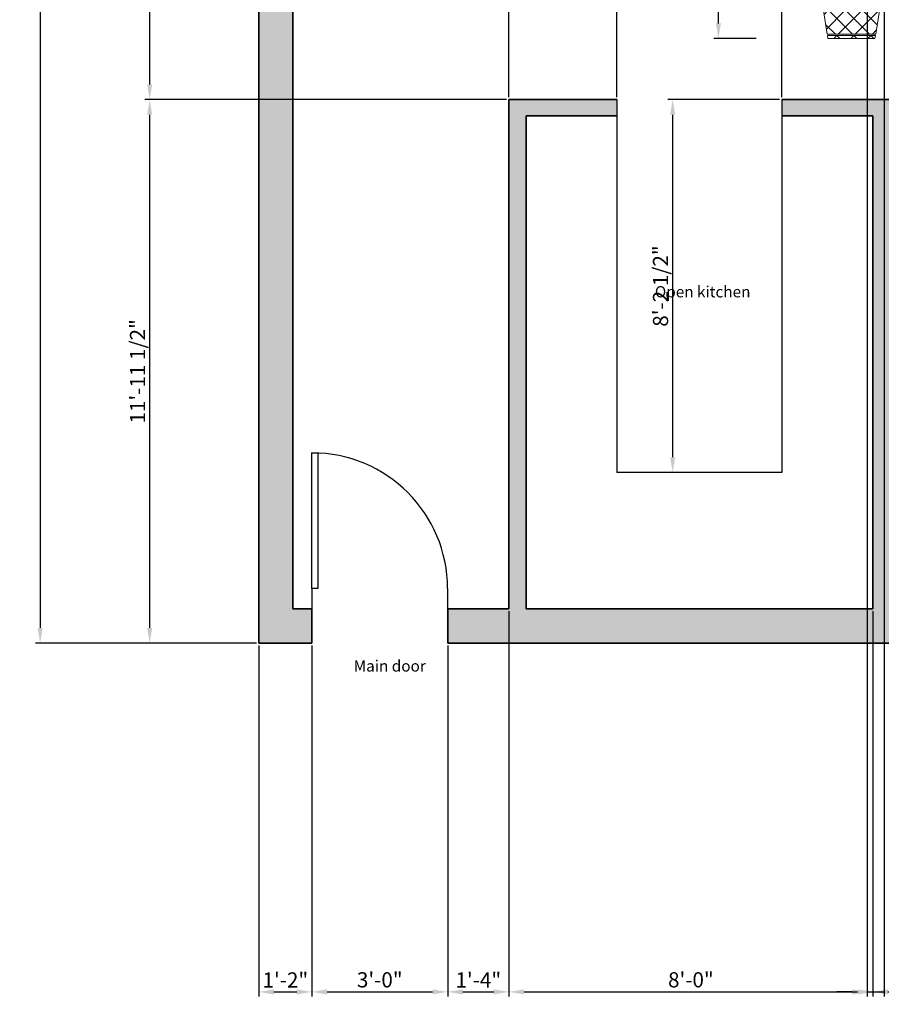
# Model space of a CAD drawing. Units: inches. Extents: x 1872 to 2380, y 714 to 1327.
# Tile 1 of 9: x 1872 to 2100, y 714 to 974. Entities that reach past the tile are written whole.
import ezdxf

# ---------------------------------------------------------------- set-up
doc = ezdxf.new("R2010")
doc.units = ezdxf.units.IN
for name, color, linetype, lineweight in [('A-ANNO-DIMS', 2, 'Continuous', 18), ('A-ANNO-TEXT', 7, 'Continuous', 18), ('A-AREA-IDEN', 7, 'Continuous', 18), ('A-DOOR', 4, 'Continuous', 25), ('A-FLOR-CASE', 8, 'Continuous', 25), ('A-FURN', 8, 'Continuous', 18), ('A-WALL', 7, 'Continuous', 35)]:
    doc.layers.add(name, color=color, linetype=linetype, lineweight=lineweight)
doc.layers.add('A-FURN-PATT', color=254, linetype='Continuous', lineweight=13, true_color=0xf8ceb3)
doc.layers.add('A-WALL-PATT', color=242, linetype='Continuous', lineweight=13, true_color=0xd52e31)
doc.styles.get("Standard").update_dxf_attribs({"font": 'arial.ttf'})
doc.dimstyles.new('ISO-25', dxfattribs={"dimtxt": 4, "dimasz": 4, "dimexe": 1.25, "dimexo": 0.625, "dimtad": 1, "dimdec": 0, "dimlunit": 3, "dimtxsty": 'Standard', "dimcen": 2.5, "dimadec": 0, "dimazin": 0, "dimtfac": 1, "dimtdec": 0, "dimtmove": 0, "dimatfit": 3, "dimfxl": 1, "dimarcsym": 0})

# ---------------------------------------------------------------- blocks, each defined once
blk = doc.blocks.new('*U3')
for p, q in [((0, 0), (0, -6)), ((40, 0), (40, -6))]:
    blk.add_line(p, q)
blk.add_lwpolyline([(0, 0), (0, 40), (1.75, 40), (1.75, 0)], close=True)
blk.add_arc((0, 0), 40, 0, 90)
blk = doc.blocks.new('Dining Set - 36 x 72 in.')
for p, q in [((-22, 27.5), (-22.1562, 26.50042)), ((-22, 27.5), (-6, 27.5)), ((-5.8437, 26.49966), (-6, 27.5)), ((6, 27.5), (5.8438, 26.50042)), ((6, 27.5), (22, 27.5)), ((22.1563, 26.49966), (22, 27.5)), ((-22.2343, 26.00059), (-23.4847, 17.99762)), ((-22.2304, 26), (-5.7608, 26)), ((-5.8416, 26.5), (-22.1534, 26.5)), ((-4.5152, 17.99762), (-5.7655, 25.99926)), ((5.7657, 26.00059), (4.5153, 17.99762)), ((5.7696, 26), (22.2392, 26)), ((22.1584, 26.5), (5.8466, 26.5)), ((23.4848, 17.99762), (22.2345, 25.99926)), ((36, 18), (-36, 18)), ((-36, 18), (-36, -18)), ((36, -18), (36, 18)), ((-45.5, 8), (-44.5004, 8.15617)), ((-45.5, 8), (-45.5, -8)), ((-44.5, -8.15843), (-44.5, 8.15338)), ((-44.0006, 8.23428), (-35.9976, 9.48474)), ((-44, 8.23041), (-44, -8.23915)), ((44.0006, 8.23428), (35.9976, 9.48474)), ((44, 8.23041), (44, -8.23915)), ((44.5, -8.15843), (44.5, 8.15338)), ((45.5, 8), (44.5005, 8.15617)), ((45.5, 8), (45.5, -8)), ((-44.4997, -8.15631), (-45.5, -8)), ((-35.9976, -9.48476), (-43.9993, -8.2345)), ((35.9976, -9.48476), (43.9993, -8.2345)), ((44.4997, -8.15631), (45.5, -8)), ((-36, -18), (36, -18)), ((-22.2343, -26.0006), (-23.4847, -17.99762)), ((-4.5152, -17.99762), (-5.7655, -25.99928)), ((5.7657, -26.0006), (4.5153, -17.99762)), ((23.4848, -17.99762), (22.2345, -25.99928)), ((-22.2304, -26), (-5.7608, -26)), ((-22, -27.5), (-22.1562, -26.50044)), ((-5.8416, -26.5), (-22.1534, -26.5)), ((-5.8437, -26.49967), (-6, -27.5)), ((5.7696, -26), (22.2392, -26)), ((6, -27.5), (5.8438, -26.50044)), ((22.1584, -26.5), (5.8466, -26.5)), ((22.1563, -26.49967), (22, -27.5)), ((-22, -27.5), (-6, -27.5)), ((6, -27.5), (22, -27.5))]:
    blk.add_line(p, q)
for points in [[(-36, 15), (-31.1772, 14.97754), (-26.8079, 14.91406), (-22.8538, 14.81543), (-19.276, 14.6875), (-16.0362, 14.53613), (-13.0957, 14.36718), (-10.4159, 14.18652), (-7.9583, 14), (-5.6904, 13.81315), (-3.6035, 13.63021), (-1.6954, 13.45508), (0.0365, 13.29166), (1.5945, 13.14388), (2.9811, 13.01562), (4.1988, 12.9108), (5.25, 12.83333), (6.1393, 12.78613), (6.8802, 12.76823), (7.4883, 12.77767), (7.9792, 12.8125), (8.3685, 12.87077), (8.6719, 12.95052), (8.9049, 13.0498), (9.0833, 13.16666), (9.2205, 13.29899), (9.3216, 13.44401), (9.3895, 13.59879), (9.4271, 13.76041), (9.4373, 13.92594), (9.4232, 14.09245), (9.3875, 14.257), (9.3333, 14.41666), (9.2638, 14.56917), (9.1836, 14.71484), (9.0975, 14.85465), (9.0104, 14.98958), (8.9272, 15.1206), (8.8529, 15.2487), (8.7922, 15.37483), (8.75, 15.5), (8.7305, 15.62467), (8.7344, 15.74739), (8.7617, 15.86621), (8.8125, 15.97916), (8.8867, 16.08431), (8.9844, 16.17968), (9.1055, 16.26334), (9.25, 16.33333), (9.4189, 16.38802), (9.6172, 16.42708), (9.8506, 16.45052), (10.125, 16.45833), (10.4463, 16.45052), (10.8203, 16.42708), (11.2529, 16.38802), (11.75, 16.33333), (12.3184, 16.26318), (12.9694, 16.17838), (13.7151, 16.07991), (14.5677, 15.96875), (15.5395, 15.84586), (16.6426, 15.71224), (17.8893, 15.56884), (19.2917, 15.41666), (20.859, 15.25667), (22.5879, 15.08984), (24.4721, 14.91715), (26.5052, 14.73958), (28.6809, 14.5581), (30.9929, 14.3737), (33.4347, 14.18733), (36, 14)], [(-36, 10), (-28.9766, 10.14274), (-23.1725, 10.20442), (-18.4241, 10.19775), (-14.5677, 10.13541), (-11.4399, 10.03011), (-8.877, 9.89453), (-6.7154, 9.74137), (-4.7917, 9.58333), (-2.9698, 9.43082), (-1.2246, 9.28515), (0.4415, 9.14534), (2.026, 9.01041), (3.5266, 8.87939), (4.9408, 8.7513), (6.266, 8.62516), (7.5, 8.5), (8.6411, 8.37549), (9.6914, 8.2539), (10.6538, 8.13818), (11.5312, 8.03125), (12.3267, 7.93603), (13.043, 7.85547), (13.6831, 7.79248), (14.25, 7.75), (14.7471, 7.7303), (15.1797, 7.73307), (15.5537, 7.75732), (15.875, 7.80208), (16.1494, 7.86637), (16.3828, 7.94922), (16.5811, 8.04964), (16.75, 8.16666), (16.8944, 8.29915), (17.0143, 8.44531), (17.1089, 8.60319), (17.1771, 8.77083), (17.218, 8.94629), (17.2305, 9.1276), (17.2137, 9.31282), (17.1667, 9.5), (17.0895, 9.6875), (16.987, 9.875), (16.8649, 10.0625), (16.7292, 10.25), (16.5856, 10.4375), (16.4401, 10.625), (16.2985, 10.8125), (16.1667, 11), (16.05, 11.18733), (15.9518, 11.3737), (15.8752, 11.5581), (15.8229, 11.73958), (15.798, 11.91715), (15.8034, 12.08984), (15.842, 12.25667), (15.9167, 12.41666), (16.0295, 12.56836), (16.1784, 12.70833), (16.3605, 12.83268), (16.5729, 12.9375), (16.8127, 13.01888), (17.0768, 13.07291), (17.3625, 13.0957), (17.6667, 13.08333), (17.9894, 13.03312), (18.3418, 12.94726), (18.7382, 12.82918), (19.1927, 12.68229), (19.7195, 12.51001), (20.3327, 12.31575), (21.0465, 12.10294), (21.875, 11.875), (22.8357, 11.63354), (23.959, 11.37304), (25.2786, 11.08618), (26.8282, 10.76562), (28.6414, 10.40405), (30.752, 9.99414), (33.1936, 9.52856), (36, 9)], [(-36, 5.5), (-30.7157, 5.3348), (-26.069, 5.20963), (-21.9946, 5.11767), (-18.4271, 5.05208), (-15.3009, 5.00602), (-12.5508, 4.97265), (-10.1112, 4.94515), (-7.9167, 4.91666), (-5.909, 4.88167), (-4.0586, 4.83984), (-2.3429, 4.79215), (-0.7396, 4.73958), (0.7739, 4.6831), (2.22, 4.6237), (3.6213, 4.56233), (5, 4.5), (6.373, 4.43782), (7.7344, 4.3776), (9.0723, 4.32129), (10.375, 4.27083), (11.6309, 4.22819), (12.8281, 4.19531), (13.9551, 4.17415), (15, 4.16666), (15.954, 4.17448), (16.819, 4.19791), (17.6001, 4.23698), (18.3021, 4.29166), (18.9299, 4.36198), (19.4883, 4.44791), (19.9823, 4.54948), (20.4167, 4.66666), (20.7969, 4.79899), (21.1302, 4.94401), (21.4245, 5.09879), (21.6875, 5.26041), (21.9271, 5.42594), (22.1511, 5.59245), (22.3672, 5.757), (22.5834, 5.91666), (22.8065, 6.06868), (23.0404, 6.21093), (23.2879, 6.34147), (23.5521, 6.45833), (23.8358, 6.55957), (24.142, 6.64323), (24.4735, 6.70735), (24.8334, 6.75), (25.2235, 6.76969), (25.642, 6.76692), (26.0858, 6.74267), (26.5521, 6.69791), (27.0379, 6.63362), (27.5404, 6.55078), (28.0565, 6.45036), (28.5834, 6.33333), (29.1242, 6.19987), (29.7071, 6.04687), (30.3661, 5.87044), (31.1354, 5.66666), (32.0493, 5.43164), (33.142, 5.16146), (34.4475, 4.85221), (36, 4.5)], [(-36, -1), (-30.7915, -0.6591), (-26.0195, -0.38216), (-21.6519, -0.16284), (-17.6563, 0.00521), (-14.0005, 0.12833), (-10.6523, 0.21289), (-7.5796, 0.26522), (-4.75, 0.29166), (-2.134, 0.29793), (0.2878, 0.28711), (2.5317, 0.26163), (4.6146, 0.22396), (6.5529, 0.17651), (8.3633, 0.12174), (10.0623, 0.06209), (11.6667, 0), (13.1899, -0.06201), (14.6341, -0.1211), (15.9982, -0.17432), (17.2813, -0.21875), (18.4823, -0.25147), (19.6003, -0.26953), (20.6343, -0.27002), (21.5834, -0.25), (22.4481, -0.20768), (23.2357, -0.14584), (23.9549, -0.06836), (24.6146, 0.02083), (25.2235, 0.11784), (25.7904, 0.21875), (26.3241, 0.31966), (26.8334, 0.41666), (27.3265, 0.50618), (27.8099, 0.58593), (28.2894, 0.65397), (28.7709, 0.70833), (29.2601, 0.74707), (29.763, 0.76823), (30.2855, 0.76985), (30.8334, 0.75), (31.4088, 0.70784), (31.9994, 0.64713), (32.589, 0.57275), (33.1615, 0.48958), (33.7008, 0.4025), (34.1908, 0.3164), (34.6153, 0.23616), (34.9584, 0.16666), (35.2099, 0.11165), (35.3848, 0.07031), (35.504, 0.04069), (35.5886, 0.02083), (35.6594, 0.00879), (35.7377, 0.0026), (35.8442, 0.00032), (36, 0)], [(-36, -6.5), (-27.1843, -6.31267), (-20.084, -6.1263), (-14.469, -5.9419), (-10.1094, -5.76042), (-6.7752, -5.58285), (-4.2363, -5.41016), (-2.2629, -5.24333), (-0.625, -5.08334), (0.8708, -4.93099), (2.2715, -4.78646), (3.5872, -4.64974), (4.8281, -4.52084), (6.0046, -4.39974), (7.127, -4.28646), (8.2053, -4.18099), (9.25, -4.08334), (10.2705, -3.99382), (11.2734, -3.91407), (12.2647, -3.84603), (13.25, -3.79167), (14.2354, -3.75293), (15.2266, -3.73177), (16.2295, -3.73015), (17.25, -3.75), (18.2912, -3.79248), (19.3451, -3.85547), (20.4009, -3.93604), (21.4479, -4.03125), (22.4754, -4.13819), (23.4727, -4.25391), (24.4289, -4.37549), (25.3334, -4.5), (26.1785, -4.62492), (26.9694, -4.74935), (27.7145, -4.87281), (28.4219, -4.99479), (29.1, -5.11483), (29.7572, -5.23242), (30.4016, -5.34709), (31.0417, -5.45834), (31.6837, -5.56437), (32.3262, -5.65821), (32.9658, -5.73153), (33.599, -5.77604), (34.2224, -5.78345), (34.8327, -5.74545), (35.4264, -5.65373), (36, -5.5)], [(-36, -10), (-26.4022, -9.81299), (-18.4675, -9.62891), (-11.9839, -9.45069), (-6.7396, -9.28125), (-2.5226, -9.12354), (0.8789, -8.98047), (3.6769, -8.85498), (6.0833, -8.75), (8.2767, -8.66765), (10.3021, -8.60677), (12.1712, -8.56543), (13.8958, -8.54167), (15.4876, -8.53353), (16.9583, -8.53907), (18.3197, -8.55632), (19.5834, -8.58334), (20.7616, -8.61841), (21.8685, -8.66081), (22.9188, -8.71004), (23.9271, -8.76563), (24.9081, -8.82707), (25.8763, -8.89388), (26.8465, -8.96558), (27.8334, -9.04167), (28.8474, -9.12118), (29.8828, -9.20117), (30.93, -9.27824), (31.9792, -9.34896), (33.0205, -9.40991), (34.0443, -9.45768), (35.0407, -9.48885), (36, -9.5)], [(-36, -14.5), (-30.0881, -14.33513), (-25.0332, -14.21224), (-20.7312, -14.12647), (-17.0781, -14.07292), (-13.97, -14.04671), (-11.3027, -14.04297), (-8.9724, -14.05681), (-6.875, -14.08334), (-4.9224, -14.11833), (-3.0905, -14.16016), (-1.3709, -14.20785), (0.2448, -14.26042), (1.7647, -14.3169), (3.1973, -14.3763), (4.5507, -14.43767), (5.8333, -14.5), (7.0554, -14.5621), (8.235, -14.62175), (9.3922, -14.67652), (10.5469, -14.72396), (11.7192, -14.76164), (12.929, -14.78711), (14.1965, -14.79794), (15.5417, -14.79167), (16.9933, -14.76424), (18.6152, -14.70508), (20.4804, -14.60197), (22.6615, -14.44271), (25.2312, -14.21509), (28.2624, -13.9069), (31.8277, -13.50594), (36, -13)]]:
    blk.add_lwpolyline(points)
blk = doc.blocks.new('*D23')
at = {"layer": 'A-ANNO-DIMS', "color": 0, "lineweight": -2, "transparency": 16777216}
for p, q in [((1934.77, 1289.64), (1876.44, 1289.64)), ((1877.69, 1285.64), (1877.69, 813.64)), ((1934.77, 809.64), (1876.44, 809.64))]:
    blk.add_line(p, q, dxfattribs=at)
at = {"layer": 'A-ANNO-DIMS', "color": 0, "transparency": 16777216}
for points in [[(1877.02, 1285.64), (1878.36, 1285.64), (1877.69, 1289.64)], [(1877.02, 813.64), (1878.36, 813.64), (1877.69, 809.64)]]:
    blk.add_solid(points, dxfattribs=at)
at = {"layer": 'Defpoints', "color": 0, "transparency": 16777216}
for p in [(1935.4, 1289.64), (1877.69, 809.64), (1935.4, 809.64)]:
    blk.add_point(p, dxfattribs=at)
at = {"layer": 'A-ANNO-DIMS', "color": 0, "transparency": 16777216, "insert": (1875.02, 1049.64), "char_height": 4, "attachment_point": 5, "rotation": 90}
blk.add_mtext("40'", dxfattribs=at)
blk = doc.blocks.new('*D47')
at = {"layer": 'A-ANNO-DIMS', "color": 0, "lineweight": -2, "transparency": 16777216}
for p, q in [((2066.65, 1011.83), (2055.42, 1011.83)), ((2056.67, 973.09), (2056.67, 1007.83)), ((2066.65, 969.09), (2055.42, 969.09))]:
    blk.add_line(p, q, dxfattribs=at)
at = {"layer": 'A-ANNO-DIMS', "color": 0, "transparency": 16777216}
for points in [[(2056, 1007.83), (2057.33, 1007.83), (2056.67, 1011.83)], [(2056, 973.09), (2057.33, 973.09), (2056.67, 969.09)]]:
    blk.add_solid(points, dxfattribs=at)
at = {"layer": 'Defpoints', "color": 0, "transparency": 16777216}
for p in [(2056.67, 1011.83), (2067.28, 1011.83), (2067.28, 969.09)]:
    blk.add_point(p, dxfattribs=at)
at = {"layer": 'A-ANNO-DIMS', "color": 0, "transparency": 16777216, "insert": (2053.97, 990.46), "char_height": 4, "attachment_point": 5, "rotation": 90}
blk.add_mtext('3\'-6 1/2"', dxfattribs=at)
blk = doc.blocks.new('*D56')
at = {"layer": 'A-ANNO-DIMS', "color": 0, "lineweight": -2, "transparency": 16777216}
for p, q in [((1935.4, 809.02), (1935.4, 716.39)), ((1949.4, 809.02), (1949.4, 716.39)), ((1939.4, 717.64), (1945.4, 717.64))]:
    blk.add_line(p, q, dxfattribs=at)
at = {"layer": 'A-ANNO-DIMS', "color": 0, "transparency": 16777216}
for points in [[(1939.4, 718.3), (1939.4, 716.97), (1935.4, 717.64)], [(1945.4, 718.3), (1945.4, 716.97), (1949.4, 717.64)]]:
    blk.add_solid(points, dxfattribs=at)
at = {"layer": 'Defpoints', "color": 0, "transparency": 16777216}
for p in [(1935.4, 809.64), (1949.4, 809.64), (1949.4, 717.64)]:
    blk.add_point(p, dxfattribs=at)
at = {"layer": 'A-ANNO-DIMS', "color": 0, "transparency": 16777216, "insert": (1942.4, 720.27), "char_height": 4, "attachment_point": 5}
blk.add_mtext('1\'-2"', dxfattribs=at)
blk = doc.blocks.new('*D57')
at = {"layer": 'A-ANNO-DIMS', "color": 0, "lineweight": -2, "transparency": 16777216}
for p, q in [((1949.4, 809.02), (1949.4, 716.39)), ((1985.23, 809.02), (1985.23, 716.39)), ((1953.4, 717.64), (1981.23, 717.64))]:
    blk.add_line(p, q, dxfattribs=at)
at = {"layer": 'A-ANNO-DIMS', "color": 0, "transparency": 16777216}
for points in [[(1953.4, 718.3), (1953.4, 716.97), (1949.4, 717.64)], [(1981.23, 718.3), (1981.23, 716.97), (1985.23, 717.64)]]:
    blk.add_solid(points, dxfattribs=at)
at = {"layer": 'Defpoints', "color": 0, "transparency": 16777216}
for p in [(1949.4, 809.64), (1985.23, 809.64), (1985.23, 717.64)]:
    blk.add_point(p, dxfattribs=at)
at = {"layer": 'A-ANNO-DIMS', "color": 0, "transparency": 16777216, "insert": (1967.31, 720.31), "char_height": 4, "attachment_point": 5}
blk.add_mtext('3\'-0"', dxfattribs=at)
blk = doc.blocks.new('*D58')
at = {"layer": 'A-ANNO-DIMS', "color": 0, "lineweight": -2, "transparency": 16777216}
for p, q in [((2001.4, 818.02), (2001.4, 716.39)), ((1985.23, 809.02), (1985.23, 716.39)), ((1989.23, 717.64), (1997.4, 717.64))]:
    blk.add_line(p, q, dxfattribs=at)
at = {"layer": 'A-ANNO-DIMS', "color": 0, "transparency": 16777216}
for points in [[(1989.23, 718.3), (1989.23, 716.97), (1985.23, 717.64)], [(1997.4, 718.3), (1997.4, 716.97), (2001.4, 717.64)]]:
    blk.add_solid(points, dxfattribs=at)
at = {"layer": 'Defpoints', "color": 0, "transparency": 16777216}
for p in [(2001.4, 818.64), (1985.23, 809.64), (2001.4, 717.64)]:
    blk.add_point(p, dxfattribs=at)
at = {"layer": 'A-ANNO-DIMS', "color": 0, "transparency": 16777216, "insert": (1993.31, 720.27), "char_height": 4, "attachment_point": 5}
blk.add_mtext('1\'-4"', dxfattribs=at)
blk = doc.blocks.new('*D59')
at = {"layer": 'A-ANNO-DIMS', "color": 0, "lineweight": -2, "transparency": 16777216}
for p, q in [((2001.4, 818.02), (2001.4, 716.39)), ((2097.4, 818.02), (2097.4, 716.39)), ((2005.4, 717.64), (2093.4, 717.64))]:
    blk.add_line(p, q, dxfattribs=at)
at = {"layer": 'A-ANNO-DIMS', "color": 0, "transparency": 16777216}
for points in [[(2005.4, 718.3), (2005.4, 716.97), (2001.4, 717.64)], [(2093.4, 718.3), (2093.4, 716.97), (2097.4, 717.64)]]:
    blk.add_solid(points, dxfattribs=at)
at = {"layer": 'Defpoints', "color": 0, "transparency": 16777216}
for p in [(2001.4, 818.64), (2097.4, 818.64), (2097.4, 717.64)]:
    blk.add_point(p, dxfattribs=at)
at = {"layer": 'A-ANNO-DIMS', "color": 0, "transparency": 16777216, "insert": (2049.4, 720.31), "char_height": 4, "attachment_point": 5}
blk.add_mtext('8\'-0"', dxfattribs=at)
blk = doc.blocks.new('*D60')
at = {"layer": 'A-ANNO-DIMS', "color": 0, "lineweight": -2, "transparency": 16777216}
for p, q in [((2097.4, 818.02), (2097.4, 716.39)), ((2197.9, 818.02), (2197.9, 716.39)), ((2101.4, 717.64), (2193.9, 717.64))]:
    blk.add_line(p, q, dxfattribs=at)
at = {"layer": 'A-ANNO-DIMS', "color": 0, "transparency": 16777216}
for points in [[(2101.4, 718.3), (2101.4, 716.97), (2097.4, 717.64)], [(2193.9, 718.3), (2193.9, 716.97), (2197.9, 717.64)]]:
    blk.add_solid(points, dxfattribs=at)
at = {"layer": 'Defpoints', "color": 0, "transparency": 16777216}
for p in [(2097.4, 818.64), (2197.9, 818.64), (2197.9, 717.64)]:
    blk.add_point(p, dxfattribs=at)
at = {"layer": 'A-ANNO-DIMS', "color": 0, "transparency": 16777216, "insert": (2147.65, 720.33), "char_height": 4, "attachment_point": 5}
blk.add_mtext('8\'-4 1/2"', dxfattribs=at)
blk = doc.blocks.new('*D66')
at = {"layer": 'A-ANNO-DIMS', "color": 0, "lineweight": -2, "transparency": 16777216}
for p, q in [((2000.77, 952.99), (1905.35, 952.99)), ((1906.6, 813.64), (1906.6, 948.99)), ((1934.77, 809.64), (1905.35, 809.64))]:
    blk.add_line(p, q, dxfattribs=at)
at = {"layer": 'A-ANNO-DIMS', "color": 0, "transparency": 16777216}
for points in [[(1905.93, 948.99), (1907.27, 948.99), (1906.6, 952.99)], [(1905.93, 813.64), (1907.27, 813.64), (1906.6, 809.64)]]:
    blk.add_solid(points, dxfattribs=at)
at = {"layer": 'Defpoints', "color": 0, "transparency": 16777216}
for p in [(1906.6, 952.99), (2001.4, 952.99), (1935.4, 809.64)]:
    blk.add_point(p, dxfattribs=at)
at = {"layer": 'A-ANNO-DIMS', "color": 0, "transparency": 16777216, "insert": (1903.91, 881.32), "char_height": 4, "attachment_point": 5, "rotation": 90}
blk.add_mtext('11\'-11 1/2"', dxfattribs=at)
blk = doc.blocks.new('*D67')
at = {"layer": 'A-ANNO-DIMS', "color": 0, "lineweight": -2, "transparency": 16777216}
for p, q in [((1943.77, 1112.77), (1905.35, 1112.77)), ((1906.6, 956.99), (1906.6, 1108.77)), ((2000.77, 952.99), (1905.35, 952.99))]:
    blk.add_line(p, q, dxfattribs=at)
at = {"layer": 'A-ANNO-DIMS', "color": 0, "transparency": 16777216}
for points in [[(1905.93, 1108.77), (1907.27, 1108.77), (1906.6, 1112.77)], [(1905.93, 956.99), (1907.27, 956.99), (1906.6, 952.99)]]:
    blk.add_solid(points, dxfattribs=at)
at = {"layer": 'Defpoints', "color": 0, "transparency": 16777216}
for p in [(1906.6, 1112.77), (1944.4, 1112.77), (2001.4, 952.99)]:
    blk.add_point(p, dxfattribs=at)
at = {"layer": 'A-ANNO-DIMS', "color": 0, "transparency": 16777216, "insert": (1903.93, 1032.88), "char_height": 4, "attachment_point": 5, "rotation": 90}
blk.add_mtext('13\'-4"', dxfattribs=at)
blk = doc.blocks.new('*D76')
at = {"layer": 'A-ANNO-DIMS', "color": 0, "lineweight": -2, "transparency": 16777216}
for p, q in [((2001.4, 953.62), (2001.4, 1319.69)), ((2029.9, 953.62), (2029.9, 1319.69)), ((2005.4, 1318.44), (2025.9, 1318.44))]:
    blk.add_line(p, q, dxfattribs=at)
at = {"layer": 'A-ANNO-DIMS', "color": 0, "transparency": 16777216}
for points in [[(2005.4, 1319.11), (2005.4, 1317.78), (2001.4, 1318.44)], [(2025.9, 1319.11), (2025.9, 1317.78), (2029.9, 1318.44)]]:
    blk.add_solid(points, dxfattribs=at)
at = {"layer": 'Defpoints', "color": 0, "transparency": 16777216}
for p in [(2029.9, 1318.44), (2001.4, 952.99), (2029.9, 952.99)]:
    blk.add_point(p, dxfattribs=at)
at = {"layer": 'A-ANNO-DIMS', "color": 0, "transparency": 16777216, "insert": (2015.65, 1321.14), "char_height": 4, "attachment_point": 5}
blk.add_mtext('2\'-4 1/2"', dxfattribs=at)
blk = doc.blocks.new('*D77')
at = {"layer": 'A-ANNO-DIMS', "color": 0, "lineweight": -2, "transparency": 16777216}
for p, q in [((2029.9, 953.62), (2029.9, 1319.69)), ((2073.4, 953.62), (2073.4, 1319.69)), ((2033.9, 1318.44), (2069.4, 1318.44))]:
    blk.add_line(p, q, dxfattribs=at)
at = {"layer": 'A-ANNO-DIMS', "color": 0, "transparency": 16777216}
for points in [[(2033.9, 1319.11), (2033.9, 1317.78), (2029.9, 1318.44)], [(2069.4, 1319.11), (2069.4, 1317.78), (2073.4, 1318.44)]]:
    blk.add_solid(points, dxfattribs=at)
at = {"layer": 'Defpoints', "color": 0, "transparency": 16777216}
for p in [(2073.4, 1318.44), (2029.9, 952.99), (2073.4, 952.99)]:
    blk.add_point(p, dxfattribs=at)
at = {"layer": 'A-ANNO-DIMS', "color": 0, "transparency": 16777216, "insert": (2051.65, 1321.14), "char_height": 4, "attachment_point": 5}
blk.add_mtext('3\'-7 1/2"', dxfattribs=at)
blk = doc.blocks.new('*D78')
at = {"layer": 'A-ANNO-DIMS', "color": 0, "lineweight": -2, "transparency": 16777216}
for p, q in [((2072.77, 952.99), (2043.35, 952.99)), ((2044.6, 858.64), (2044.6, 948.99)), ((2072.77, 854.64), (2043.35, 854.64))]:
    blk.add_line(p, q, dxfattribs=at)
at = {"layer": 'A-ANNO-DIMS', "color": 0, "transparency": 16777216}
for points in [[(2043.93, 948.99), (2045.27, 948.99), (2044.6, 952.99)], [(2043.93, 858.64), (2045.27, 858.64), (2044.6, 854.64)]]:
    blk.add_solid(points, dxfattribs=at)
at = {"layer": 'Defpoints', "color": 0, "transparency": 16777216}
for p in [(2044.6, 952.99), (2073.4, 952.99), (2073.4, 854.64)]:
    blk.add_point(p, dxfattribs=at)
at = {"layer": 'A-ANNO-DIMS', "color": 0, "transparency": 16777216, "insert": (2041.91, 903.82), "char_height": 4, "attachment_point": 5, "rotation": 90}
blk.add_mtext('8\'-2 1/2"', dxfattribs=at)
blk = doc.blocks.new('*D80')
at = {"layer": 'A-ANNO-DIMS', "color": 0, "lineweight": -2, "transparency": 16777216}
for p, q in [((2095.9, 1112.15), (2095.9, 716.39)), ((2100.4, 1112.15), (2100.4, 716.39)), ((2091.9, 717.64), (2087.9, 717.64)), ((2095.9, 717.64), (2100.4, 717.64)), ((2104.4, 717.64), (2129.6, 717.64))]:
    blk.add_line(p, q, dxfattribs=at)
at = {"layer": 'A-ANNO-DIMS', "color": 0, "transparency": 16777216}
for points in [[(2091.9, 718.3), (2091.9, 716.97), (2095.9, 717.64)], [(2104.4, 718.3), (2104.4, 716.97), (2100.4, 717.64)]]:
    blk.add_solid(points, dxfattribs=at)
at = {"layer": 'Defpoints', "color": 0, "transparency": 16777216}
for p in [(2095.9, 1112.77), (2100.4, 1112.77), (2100.4, 717.64)]:
    blk.add_point(p, dxfattribs=at)
at = {"layer": 'A-ANNO-DIMS', "color": 0, "transparency": 16777216, "insert": (2119, 720.33), "char_height": 4, "attachment_point": 5}
blk.add_mtext('0\'-4 1/2"', dxfattribs=at)

msp = doc.modelspace()

# ---------------------------------------------------------------- hatches: boundary and pattern name
at = {"layer": 'A-FURN-PATT', "transparency": 33554687}
h = msp.add_hatch(dxfattribs=at)
h.set_pattern_fill('ANSI37', color=256)
h.paths.add_polyline_path([(2030.37, 1262.04), (1979.97, 1262.04), (1979.97, 1246.84), (1967.17, 1246.84), (1967.17, 1202.04), (2030.37, 1202.04)])
h.paths.add_polyline_path([(1964.77, 1246.84), (1966.77, 1248.84), (1966.77, 1254.04), (1951.57, 1254.04), (1951.57, 1233.24), (1964.77, 1233.24)])
h.paths.add_polyline_path([(1964.77, 1230.84), (1951.57, 1230.84), (1951.57, 1210.04), (1964.77, 1210.04)])
h.paths.add_polyline_path([(2268.08, 1263.68), (2221.12, 1263.68), (2221.12, 1219.09), (2258.57, 1219.09), (2258.57, 1230.39), (2268.08, 1230.39)])
h.paths.add_polyline_path([(2279.67, 1257.73), (2269.86, 1257.73), (2269.86, 1242.28), (2279.67, 1242.28)])
h.paths.add_polyline_path([(2279.67, 1240.49), (2269.86, 1240.49), (2269.86, 1230.39), (2268.38, 1228.9), (2268.38, 1225.04), (2279.67, 1225.04)])
h.paths.add_polyline_path([(2097.97, 1011.83), (2085.54, 1011.83), (2085.42, 1011.06), (2098.09, 1011.06)])
h.paths.add_polyline_path([(2098.15, 1010.67), (2085.36, 1010.67), (2084.39, 1004.45), (2099.13, 1004.45)])
h.paths.add_polyline_path([(2119.91, 1010.67), (2107.12, 1010.67), (2106.14, 1004.45), (2120.89, 1004.45)])
h.paths.add_polyline_path([(2119.73, 1011.83), (2107.3, 1011.83), (2107.18, 1011.06), (2119.85, 1011.06)])
h.paths.add_polyline_path([(2074.66, 997.83), (2068.44, 996.86), (2068.44, 984.06), (2074.66, 983.09)])
h.paths.add_polyline_path([(2068.05, 996.8), (2067.28, 996.68), (2067.28, 984.25), (2068.05, 984.12)])
h.paths.add_polyline_path([(2136.83, 996.86), (2130.61, 997.83), (2130.61, 983.09), (2136.83, 984.06)])
h.paths.add_polyline_path([(2137.99, 996.68), (2137.22, 996.8), (2137.22, 984.12), (2137.99, 984.25)])
h.paths.add_polyline_path([(2099.13, 976.47), (2084.39, 976.47), (2085.36, 970.26), (2098.15, 970.26)])
h.paths.add_polyline_path([(2120.89, 976.47), (2106.14, 976.47), (2107.12, 970.26), (2119.91, 970.26)])
h.paths.add_polyline_path([(2119.85, 969.87), (2107.18, 969.87), (2107.3, 969.09), (2119.73, 969.09)])
h.paths.add_polyline_path([(2098.09, 969.87), (2085.42, 969.87), (2085.54, 969.09), (2097.97, 969.09)])
at = {"layer": 'A-WALL-PATT', "transparency": 33554687}
h = msp.add_hatch(color=256, dxfattribs=at)
h.dxf.hatch_style = 1
h.paths.add_polyline_path([(2295.4, 1289.64), (1935.4, 1289.64), (1935.4, 809.64), (1949.4, 809.64), (1949.4, 818.64), (1944.4, 818.64), (1944.4, 1108.27), (2100.4, 1108.27), (2100.4, 1112.77), (1944.4, 1112.77), (1944.4, 1280.64), (2095.9, 1280.64), (2095.9, 1141.77), (2100.4, 1141.77), (2100.4, 1280.64), (2169.91, 1280.64), (2169.91, 1244.64), (2169.91, 1160.49, -0.053008), (2170.04, 1158.75, -0.03687), (2169.91, 1157.54), (2169.91, 1148.64), (2167.91, 1148.64), (2138.4, 1148.64), (2138.4, 1144.14), (2167.91, 1144.14), (2174.41, 1144.14), (2174.41, 1280.64), (2197.9, 1280.64), (2197.9, 1184.64), (2202.4, 1184.64), (2202.4, 1280.64), (2286.4, 1280.64), (2286.4, 1148.64), (2197.9, 1148.64), (2197.9, 1108.14), (2202.4, 1108.14), (2202.4, 1144.14), (2286.4, 1144.14), (2286.4, 1060.14), (2202.4, 1060.14), (2202.4, 1108.14), (2197.9, 1108.14), (2197.9, 1060.14), (2197.9, 1053.64), (2202.4, 1053.64), (2202.4, 1055.64), (2286.4, 1055.64), (2286.4, 976.14), (2202.4, 976.14), (2202.4, 1015.64), (2197.9, 1015.64), (2197.9, 971.64), (2197.9, 952.99), (2197.9, 818.64), (2101.9, 818.64), (2101.9, 948.71), (2130.4, 948.71), (2130.4, 952.99), (2073.4, 952.99), (2073.4, 948.71), (2097.4, 948.71), (2097.4, 818.64), (2005.9, 818.64), (2005.9, 948.71), (2029.9, 948.71), (2029.9, 952.99), (2001.4, 952.99), (2001.4, 818.64), (1996.4, 818.64), (1985.23, 818.64), (1985.23, 809.64), (1996.4, 809.64), (2295.4, 809.64)])
h.paths.add_polyline_path([(2202.4, 971.64), (2286.4, 971.64), (2286.4, 858.19), (2286.62, 858.19), (2286.62, 857.19), (2286.4, 857.19), (2286.4, 828.68), (2286.48, 828.76), (2286.4, 828.43), (2286.4, 818.64), (2256.29, 818.64), (2255.29, 818.39), (2254.54, 818.64), (2238.99, 818.64), (2238.75, 818.58), (2238.56, 818.64), (2202.4, 818.64), (2202.4, 952.99)], flags=16)
h.paths.add_polyline_path([(2260.41, 970, -0.15), (2280.41, 970), (2278.41, 967, 0.001913), (2277.92, 967.06), (2277.41, 964.5), (2278.64, 964.5), (2278.72, 964), (2279.41, 964), (2282.41, 953, -0.541163), (2280.76, 950.93), (2280.91, 950, -0.414214), (2279.91, 949), (2279.41, 949), (2279.91, 945), (2278.41, 945), (2277.91, 949), (2270.41, 949), (2262.91, 949), (2262.41, 945), (2260.91, 945), (2261.41, 949), (2260.91, 949, -0.414214), (2259.91, 950), (2260.05, 950.93, -0.505809), (2258.36, 952.83), (2261.41, 964), (2262.1, 964), (2262.17, 964.5), (2263.41, 964.5), (2262.9, 967.06, 0.001913), (2262.41, 967)], flags=0)
h.paths.add_polyline_path([(2257.85, 934.42), (2280.51, 934.42, -0.333333), (2281.77, 933.16), (2281.77, 923.09, -0.333333), (2280.51, 921.83), (2277.57, 921.83), (2277.57, 921.41), (2275.89, 921.41), (2275.89, 921.83), (2262.46, 921.83), (2262.46, 921.41), (2260.79, 921.41), (2260.79, 921.83), (2257.85, 921.83, -0.333333), (2256.59, 923.09), (2256.59, 933.16, -0.333333)], flags=0)
h.paths.add_polyline_path([(2260.61, 912.79), (2262.11, 912.79), (2262.61, 908.79), (2270.11, 908.79), (2277.61, 908.79), (2278.11, 912.79), (2279.61, 912.79), (2279.11, 908.79), (2279.61, 908.79, -0.414214), (2280.61, 907.79), (2280.46, 906.86, -0.505809), (2282.15, 904.96), (2279.11, 893.79), (2278.42, 893.79), (2278.34, 893.29), (2277.11, 893.29), (2277.62, 890.73, 0.001913), (2278.11, 890.79), (2280.11, 887.79, -0.15), (2260.11, 887.79), (2262.11, 890.79, 0.001913), (2262.59, 890.73), (2263.11, 893.29), (2261.87, 893.29), (2261.79, 893.79), (2261.11, 893.79), (2258.11, 904.79, -0.541163), (2259.75, 906.86), (2259.61, 907.79, -0.414214), (2260.61, 908.79), (2261.11, 908.79)], flags=0)
h.paths.add_polyline_path([(2252.62, 864.69), (2253.62, 864.69), (2253.62, 862.19), (2253.62, 860.69), (2256.62, 859.69, -0.362186), (2259.62, 862.19, -0.174416), (2262.62, 860.69, 0.103487), (2265.62, 859.19, -0.219276), (2266.55, 858.19), (2268.62, 858.19), (2268.62, 859.69), (2267.62, 859.69), (2267.62, 863.69), (2270.12, 863.69), (2270.12, 859.69), (2269.12, 859.69), (2269.12, 858.19), (2274.62, 858.19), (2278.62, 858.19), (2278.62, 862.69), (2275.62, 864.69), (2275.62, 865.69), (2279.62, 862.69), (2279.62, 858.19), (2279.62, 852.69), (2275.62, 849.19), (2275.62, 850.19), (2278.62, 852.69), (2278.62, 857.19), (2274.62, 857.19), (2271.12, 857.19), (2271.12, 855.69), (2272.12, 855.69), (2272.12, 851.69), (2269.62, 851.69), (2269.62, 855.69), (2270.62, 855.69), (2270.62, 857.19), (2266.55, 857.19, -0.219162), (2265.62, 856.19, 0.103506), (2262.62, 854.69, -0.174459), (2259.62, 853.19, -0.362114), (2256.62, 855.69), (2253.62, 854.69), (2253.62, 850.69), (2252.62, 850.69)], flags=0)
h.paths.add_polyline_path([(2253.62, 859.69), (2256.62, 858.69), (2256.62, 856.69), (2253.62, 855.69)], flags=0)
h.paths.add_polyline_path([(2208.62, 838.17), (2208.28, 836.61), (2207.75, 836.18), (2207.67, 833.93), (2208.71, 832.96), (2211.55, 836.09), (2214.43, 837.53), (2214.45, 837.55), (2214.61, 836.16), (2215.48, 834.9), (2215.87, 835.13), (2217.12, 836.79), (2216.83, 834.17), (2218.8, 828.76), (2219.23, 829.13), (2220.06, 831.53), (2219.5, 837.61), (2219.53, 837.66), (2219.68, 838.72), (2219.62, 838.91), (2219.72, 839.01), (2219.51, 837.47), (2219.77, 834.68), (2220.87, 834.05), (2221.03, 834.58), (2222.05, 835.47), (2222.71, 834.65), (2223.67, 836.89), (2224.63, 836.57), (2226.23, 835.08), (2227.55, 836.18), (2227.59, 837.16), (2228.42, 838.17), (2228.08, 836.61), (2227.55, 836.18), (2227.47, 833.93), (2228.51, 832.96), (2231.35, 836.09), (2234.23, 837.53), (2234.25, 837.55), (2234.42, 836.16), (2235.28, 834.9), (2235.67, 835.13), (2236.93, 836.79), (2236.93, 836.84), (2238.69, 834.65), (2239.41, 836.34), (2239.3, 837.61), (2239.34, 837.66), (2239.48, 838.72), (2239.42, 838.91), (2239.52, 839.01), (2239.31, 837.47), (2239.36, 836.98), (2240.61, 836.57), (2242.2, 835.08), (2243.53, 836.18), (2243.57, 837.16), (2244.39, 838.17), (2244.05, 836.61), (2243.53, 836.18), (2243.44, 833.93), (2244.49, 832.96), (2247.33, 836.09), (2250.21, 837.53), (2250.22, 837.55), (2250.39, 836.16), (2251.25, 834.9), (2251.65, 835.13), (2252.9, 836.79), (2252.61, 834.17), (2254.09, 830.08), (2254.54, 829.37), (2254.85, 828.99), (2255.01, 829.13), (2255.83, 831.53), (2255.29, 837.44), (2255.28, 837.44), (2255.46, 838.72), (2255.4, 838.91), (2255.5, 839.01), (2255.28, 837.47), (2255.29, 837.44), (2257.9, 836.57), (2259.5, 835.08), (2260.82, 836.18), (2260.86, 837.16), (2261.69, 838.17), (2261.35, 836.61), (2260.82, 836.18), (2260.74, 833.93), (2261.78, 832.96), (2264.62, 836.09), (2267.5, 837.53), (2267.52, 837.55), (2267.68, 836.16), (2268.54, 834.9), (2268.94, 835.13), (2270.19, 836.79), (2269.9, 834.17), (2271.79, 828.96), (2271.98, 828.86), (2272.3, 829.13), (2273.13, 831.53), (2272.56, 837.61), (2272.6, 837.66), (2272.75, 838.72), (2272.69, 838.91), (2272.79, 839.01), (2272.58, 837.47), (2273.13, 831.53), (2273.02, 831.22), (2273.67, 831.01), (2273.92, 831.6), (2273.83, 830.95), (2274.1, 830.86), (2275.75, 833.35), (2276.03, 831.86), (2276.57, 831.38), (2277, 831.91), (2277.3, 833.27), (2279.06, 830.44), (2281.09, 831.46), (2281.1, 831.48), (2281.21, 830.5), (2281.82, 829.61), (2282.1, 829.77), (2282.98, 830.94), (2282.77, 829.1), (2284.15, 825.3), (2284.46, 825.55), (2285.04, 827.24), (2284.64, 831.51), (2284.67, 831.55), (2284.77, 832.3), (2284.73, 832.43), (2284.8, 832.5), (2284.65, 831.42), (2285.04, 827.24), (2284.46, 825.55), (2283.45, 824.71), (2281.76, 819.99), (2278.73, 818.64), (2276.7, 819.65), (2275.69, 821.34), (2274.34, 822.01), (2272.32, 824.04), (2269.58, 824.33), (2268.46, 821.21), (2264.14, 819.29), (2261.26, 820.73), (2259.82, 823.13), (2257.9, 824.09), (2255.02, 826.97), (2253.29, 827.15), (2251.17, 821.21), (2246.85, 819.29), (2243.97, 820.73), (2242.53, 823.13), (2240.61, 824.09), (2237.73, 826.97), (2237.27, 827.01), (2235.19, 821.21), (2230.87, 819.29), (2227.99, 820.73), (2226.55, 823.13), (2224.63, 824.09), (2221.75, 826.97), (2217.61, 827.41), (2215.39, 821.21), (2211.07, 819.29), (2208.19, 820.73), (2206.75, 823.13), (2204.83, 824.09), (2203.87, 826.49), (2202.91, 830.81), (2202.91, 834.65), (2203.87, 836.89), (2204.83, 836.57), (2206.43, 835.08), (2207.75, 836.18), (2207.79, 837.16)], flags=0)
h.paths.add_polyline_path([(2221.04, 832.88), (2221.82, 832.52), (2222.11, 833.69), (2222.71, 834.29), (2222.71, 832.11), (2225.59, 830.81), (2226.55, 830.81), (2228.95, 822.65), (2230.87, 820.25), (2230.87, 819.29), (2233.27, 821.21), (2233.75, 823.61), (2232.79, 826.97), (2231.99, 830.19), (2236.41, 827.71), (2236.63, 831.29), (2235.93, 834.58), (2242.53, 830.81), (2241.57, 830.81), (2240.97, 831.07), (2240.47, 830.33), (2239.06, 829.14), (2239.65, 826.49), (2237.25, 829.37), (2236.52, 829.55), (2236.41, 827.71), (2231.99, 830.19), (2232.79, 826.97), (2233.75, 823.61), (2233.27, 821.21), (2230.87, 819.29), (2230.87, 820.25), (2228.95, 822.65), (2226.55, 830.81), (2225.59, 830.81), (2222.71, 832.11), (2222.71, 830.81), (2223.67, 826.49), (2221.27, 829.37), (2220.67, 830.33), (2220.67, 830.33)], flags=0)
h.paths.add_polyline_path([(2255.98, 833), (2259.82, 830.81), (2258.86, 830.81), (2257.25, 831.54), (2256.45, 830.33), (2256.66, 831.81), (2256.02, 832.1), (2255.98, 831.99)], flags=0)
h.paths.add_polyline_path([(2275.69, 826.73), (2277.07, 828.25), (2275.46, 829.74), (2276.39, 830.51), (2276.33, 828.93), (2279.06, 826.4), (2278.73, 823.36), (2277.38, 821)], flags=0)
h.paths.add_polyline_path([(2260.6, 925.25), (2276.34, 925.25), (2276.34, 931.01), (2260.6, 931.01)], flags=8)
h.paths.add_polyline_path([(2202.72, 1070.05), (2202.72, 1092.72), (2197.34, 1092.72), (2197.34, 1070.05)], flags=25)

# ---------------------------------------------------------------- linework, layer by layer
at = {"layer": 'A-FLOR-CASE', "transparency": 33554687}
for p, q in [((2029.9, 952.99), (2029.9, 854.64)), ((2073.4, 952.99), (2073.4, 854.64)), ((2073.4, 854.64), (2029.9, 854.64))]:
    msp.add_line(p, q, dxfattribs=at)
at = {"layer": 'A-WALL'}
for p, q in [((1944.4, 818.64), (1944.4, 1108.27)), ((2001.4, 952.99), (2001.4, 818.64)), ((2005.9, 948.71), (2005.9, 818.64)), ((2005.9, 948.71), (2029.9, 948.71)), ((2097.4, 948.71), (2097.4, 818.64))]:
    msp.add_line(p, q, dxfattribs=at)
at = {"layer": 'A-WALL', "transparency": 33554687}
for p, q in [((2029.9, 952.99), (2001.4, 952.99)), ((2130.4, 952.99), (2073.4, 952.99)), ((2073.4, 948.71), (2097.4, 948.71)), ((1949.4, 818.64), (1944.4, 818.64)), ((1949.4, 809.64), (1949.4, 818.64)), ((1985.23, 809.64), (1985.23, 818.64)), ((1985.23, 818.64), (1996.4, 818.64)), ((2001.4, 818.64), (1996.4, 818.64)), ((2097.4, 818.64), (2005.9, 818.64)), ((1996.4, 809.64), (1985.23, 809.64))]:
    msp.add_line(p, q, dxfattribs=at)
msp.add_lwpolyline([(1949.4, 809.64), (1935.4, 809.64), (1935.4, 1289.64), (2295.4, 1289.64), (2295.4, 809.64), (1996.4, 809.64)], dxfattribs=at)

# ---------------------------------------------------------------- block references
at = {"layer": 'A-DOOR', "xscale": 0.895133583936691, "yscale": 0.895133583936691, "zscale": 0.895133583936691}
msp.add_blockref('*U3', (1949.4, 824.01), dxfattribs=at)
at = {"layer": 'A-FURN', "transparency": 33554687, "xscale": 0.7771303306467578, "yscale": 0.7771303306467578, "zscale": 0.7771303306467578}
msp.add_blockref('Dining Set - 36 x 72 in.', (2102.64, 990.46), dxfattribs=at)

# ---------------------------------------------------------------- texts
at = {"layer": 'A-ANNO-TEXT', "transparency": 33554687}
msp.add_text('Main door ', height=2.965, dxfattribs=at).set_placement((1960.43, 802.13))
at = {"layer": 'A-AREA-IDEN', "transparency": 33554687}
msp.add_text('Open kitchen', height=2.965, dxfattribs=at).set_placement((2039.9, 900.83))

# ---------------------------------------------------------------- dimensions: what is measured, and where the dimension line sits
at = {"layer": 'A-ANNO-DIMS', "transparency": 33554687}
for base, p1, p2, picture, middle in [((2029.9, 1318.44), (2001.4, 952.99), (2029.9, 952.99), '*D76', (2015.65, 1321.14)), ((2073.4, 1318.44), (2029.9, 952.99), (2073.4, 952.99), '*D77', (2051.65, 1321.14)), ((2100.4, 717.64), (2095.9, 1112.77), (2100.4, 1112.77), '*D80', (2119, 720.33)), ((2001.4, 717.64), (1985.23, 809.64), (2001.4, 818.64), '*D58', (1993.31, 720.27)), ((2097.4, 717.64), (2001.4, 818.64), (2097.4, 818.64), '*D59', (2049.4, 720.31)), ((2197.9, 717.64), (2097.4, 818.64), (2197.9, 818.64), '*D60', (2147.65, 720.33)), ((1949.4, 717.64), (1935.4, 809.64), (1949.4, 809.64), '*D56', (1942.4, 720.27)), ((1985.23, 717.64), (1949.4, 809.64), (1985.23, 809.64), '*D57', (1967.31, 720.31))]:
    dim = msp.add_linear_dim(base=base, p1=p1, p2=p2, dimstyle='ISO-25', override={"dimdec": 1, "dimlfac": 1, "dimrnd": 0, "dimzin": 1, "dimdsep": 46, "dimlunit": 4, "dimfrac": 2}, dxfattribs=at)
    dim.commit()
    dim.dimension.update_dxf_attribs({"geometry": picture, "text_midpoint": middle})
for base, p1, p2, override, picture, middle in [((1877.69, 809.64), (1935.4, 1289.64), (1935.4, 809.64), {"dimclrd": 0, "dimclre": 0, "dimclrt": 0}, '*D23', (1875.02, 1049.64)), ((1906.6, 1112.77), (2001.4, 952.99), (1944.4, 1112.77), {"dimdec": 1, "dimlfac": 1, "dimrnd": 0, "dimzin": 1, "dimdsep": 46, "dimlunit": 4, "dimfrac": 2}, '*D67', (1903.93, 1032.88)), ((2056.67, 1011.83), (2067.28, 969.09), (2067.28, 1011.83), {"dimdec": 1, "dimlfac": 1, "dimrnd": 0, "dimzin": 1, "dimdsep": 46, "dimlunit": 4, "dimfrac": 2}, '*D47', (2053.97, 990.46)), ((1906.5987, 952.9946), (1935.3987, 809.6418), (2001.3987, 952.9946), {"dimdec": 1, "dimlfac": 1, "dimrnd": 0, "dimzin": 1, "dimdsep": 46, "dimlunit": 4, "dimfrac": 2}, '*D66', (1903.9054, 881.3182)), ((2044.5987, 952.9946), (2073.3987, 854.6418), (2073.3987, 952.9946), {"dimdec": 1, "dimlfac": 1, "dimrnd": 0, "dimzin": 1, "dimdsep": 46, "dimlunit": 4, "dimfrac": 2}, '*D78', (2041.9054, 903.8182))]:
    dim = msp.add_linear_dim(base=base, p1=p1, p2=p2, angle=90, dimstyle='ISO-25', override=override, dxfattribs=at)
    dim.commit()
    dim.dimension.update_dxf_attribs({"geometry": picture, "text_midpoint": middle})

doc.saveas('drawing.dxf')
